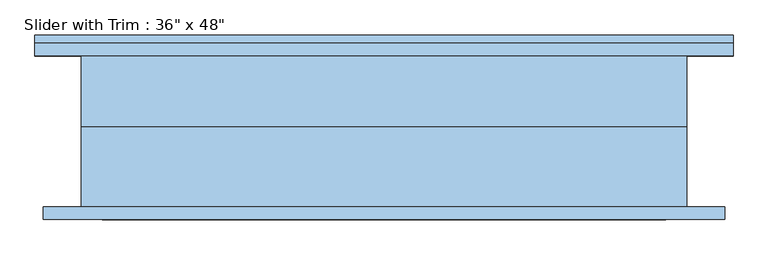
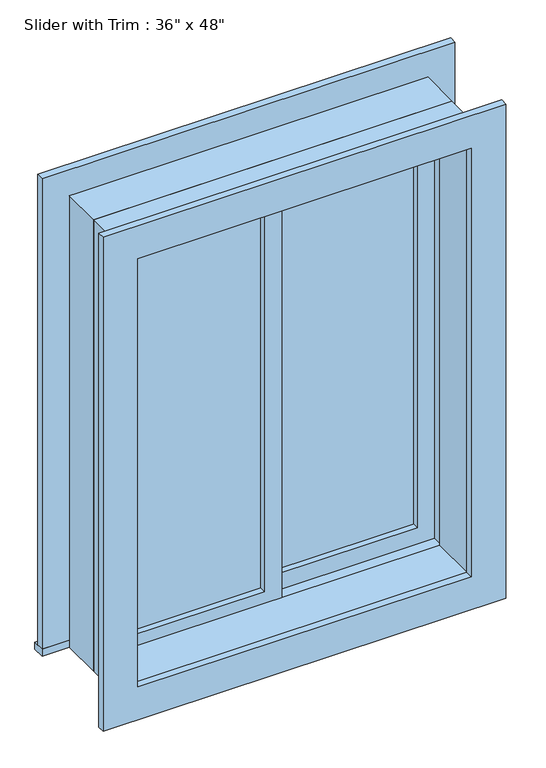
"""IFC4 building model written with IfcOpenShell, lengths in millimetres: window geometry."""

from ifc_helpers import new_model, si_unit, frame, origin, place, context, project, spatial, polyline, outline, extrude, source, transform, mapped, element, save


def window_e25db5b6(model_context):
    return source(origin(), model_context, "Body", "SweptSolid", [
        extrude(outline(polyline([(-393.7, 34.925), (-22.225, 34.925), (-22.225, 22.225), (-393.7, 22.225), (-393.7, 34.925)])), frame((0.0, 0.0, 977.9), z_axis=(0.0, 0.0, 1.0), x_axis=(1.0, 0.0, 0.0)), (0.0, 0.0, 1.0), 1092.2),
        extrude(outline(polyline([(2114.55, -438.15), (933.45, -438.15), (933.45, 22.225), (2114.55, 22.225), (2114.55, -438.15)]), holes=[polyline([(2070.1, -393.7), (2070.1, -22.225), (977.9, -22.225), (977.9, -393.7), (2070.1, -393.7)])]), frame((0.0, 6.35, 0.0), z_axis=(0.0, 1.0, 0.0), x_axis=(0.0, 0.0, 1.0)), (0.0, 0.0, 1.0), 44.45),
        extrude(outline(polyline([(-527.05, 146.05), (527.05, 146.05), (527.05, 114.3), (-527.05, 114.3), (-527.05, 146.05)])), frame((0.0, 0.0, 914.4), z_axis=(0.0, 0.0, 1.0), x_axis=(1.0, 0.0, 0.0)), (0.0, 0.0, 1.0), 19.05),
        extrude(outline(polyline([(2114.55, -438.15), (2114.55, 438.15), (933.45, 438.15), (933.45, 527.05), (2203.45, 527.05), (2203.45, -527.05), (933.45, -527.05), (933.45, -438.15), (2114.55, -438.15)])), frame((0.0, 114.3, 0.0), z_axis=(0.0, 1.0, 0.0), x_axis=(0.0, 0.0, 1.0)), (0.0, 0.0, 1.0), 19.05),
        extrude(outline(polyline([(2190.75, 514.35), (2190.75, -514.35), (857.25, -514.35), (857.25, 514.35), (2190.75, 514.35)]), holes=[polyline([(2101.85, 425.45), (946.15, 425.45), (946.15, -425.45), (2101.85, -425.45), (2101.85, 425.45)])]), frame((0.0, -133.35, 0.0), z_axis=(0.0, 1.0, 0.0), x_axis=(0.0, 0.0, 1.0)), (0.0, 0.0, 1.0), 19.05),
        extrude(outline(polyline([(393.7, 66.675), (22.225, 66.675), (22.225, 79.375), (393.7, 79.375), (393.7, 66.675)])), frame((0.0, 0.0, 977.9), z_axis=(0.0, 0.0, 1.0), x_axis=(1.0, 0.0, 0.0)), (0.0, 0.0, 1.0), 1092.2),
        extrude(outline(polyline([(2114.55, -22.225), (933.45, -22.225), (933.45, 438.15), (2114.55, 438.15), (2114.55, -22.225)]), holes=[polyline([(2070.1, 22.225), (2070.1, 393.7), (977.9, 393.7), (977.9, 22.225), (2070.1, 22.225)])]), frame((0.0, 50.8, 0.0), z_axis=(0.0, 1.0, 0.0), x_axis=(0.0, 0.0, 1.0)), (0.0, 0.0, 1.0), 44.45),
        extrude(outline(polyline([(2133.6, -457.2), (914.4, -457.2), (914.4, 457.2), (2133.6, 457.2), (2133.6, -457.2)]), holes=[polyline([(2101.85, -425.45), (2101.85, 425.45), (946.15, 425.45), (946.15, -425.45), (2101.85, -425.45)])]), frame((0.0, -114.3, 0.0), z_axis=(0.0, 1.0, 0.0), x_axis=(0.0, 0.0, 1.0)), (0.0, 0.0, 1.0), 120.65),
        extrude(outline(polyline([(2133.6, 457.2), (2133.6, -457.2), (914.4, -457.2), (914.4, 457.2), (2133.6, 457.2)]), holes=[polyline([(2114.55, 438.15), (933.45, 438.15), (933.45, -438.15), (2114.55, -438.15), (2114.55, 438.15)])]), frame((0.0, 6.35, 0.0), z_axis=(0.0, 1.0, 0.0), x_axis=(0.0, 0.0, 1.0)), (0.0, 0.0, 1.0), 107.95),
    ])


if __name__ == "__main__":
    model = new_model("IFC4")
    model_context = context("Model", 3, world=origin())
    ifc_project = project(units=[si_unit("LENGTHUNIT", "METRE", prefix="MILLI")], contexts=[model_context])
    site = spatial("IfcSite", under=ifc_project)
    building = spatial("IfcBuilding", under=site)
    placement = place(None, origin())
    window_shape = window_e25db5b6(model_context)
    element("IfcWindow", 1, ObjectType="Slider with Trim : 36\" x 48\"", at=placement, inside=building, context=model_context, shape_type="MappedRepresentation", body=[
        mapped(window_shape, transform((0.0, 0.0, 0.0), x_axis=(1.0, 0.0, 0.0), y_axis=(0.0, 1.0, 0.0), z_axis=(0.0, 0.0, 1.0))),
    ])
    save(model, "model.ifc")

# Revit data of these elements
# Type "Slider with Trim : 36\" x 48\""
#   Type Mark = "10"
#   Construction Type Id = "GSP4R"
#   Assembly Code = "B2020100"
#   Analytic Construction = "1/8 in Pilkington single glazing"
#   Visual Light Transmittance = 0.9
#   Solar Heat Gain Coefficient = 0.78
#   Heat Transfer Coefficient (U) = 0.6496 BTU/(h·ft²·°F)
#   Height = 4' - 0"
#   Default Sill Height = 3' - 0"
#   Trim Projection - Ext. = 0' - 0 3/4"
#   Trim Projection - Int. = 0' - 0 3/4"
#   Trim Width - Exterior = 0' - 3 1/2"
#   Trim Width - Interior = 0' - 3 1/2"
#   Width = 3' - 0"
#   Window Inset = 0' - 0 3/4"
#   Define Thermal Properties by = 1
#   Glass Pane Material = Glass
#   Sash Material = Sash
#   Trim Exterior Material = Trim
#   Trim Interior Material = Trim
#   Wall Closure = (empty or 0)
# Element 1 (IfcWindow, "Slider with Trim : 36\" x 48\"")
#   Materials on its faces: "Sash", "Trim", "Glass"
# Materials
#   "Glass": class "Glass", colour RGB 0 128 192, transparency 0.75, Description = "Soda Lime Glass", Cost = 0
#   "Sash": class "Wood", colour RGB 224 178 126, transparency 0
#   "Trim": class "Wood", colour RGB 224 178 126, transparency 0
